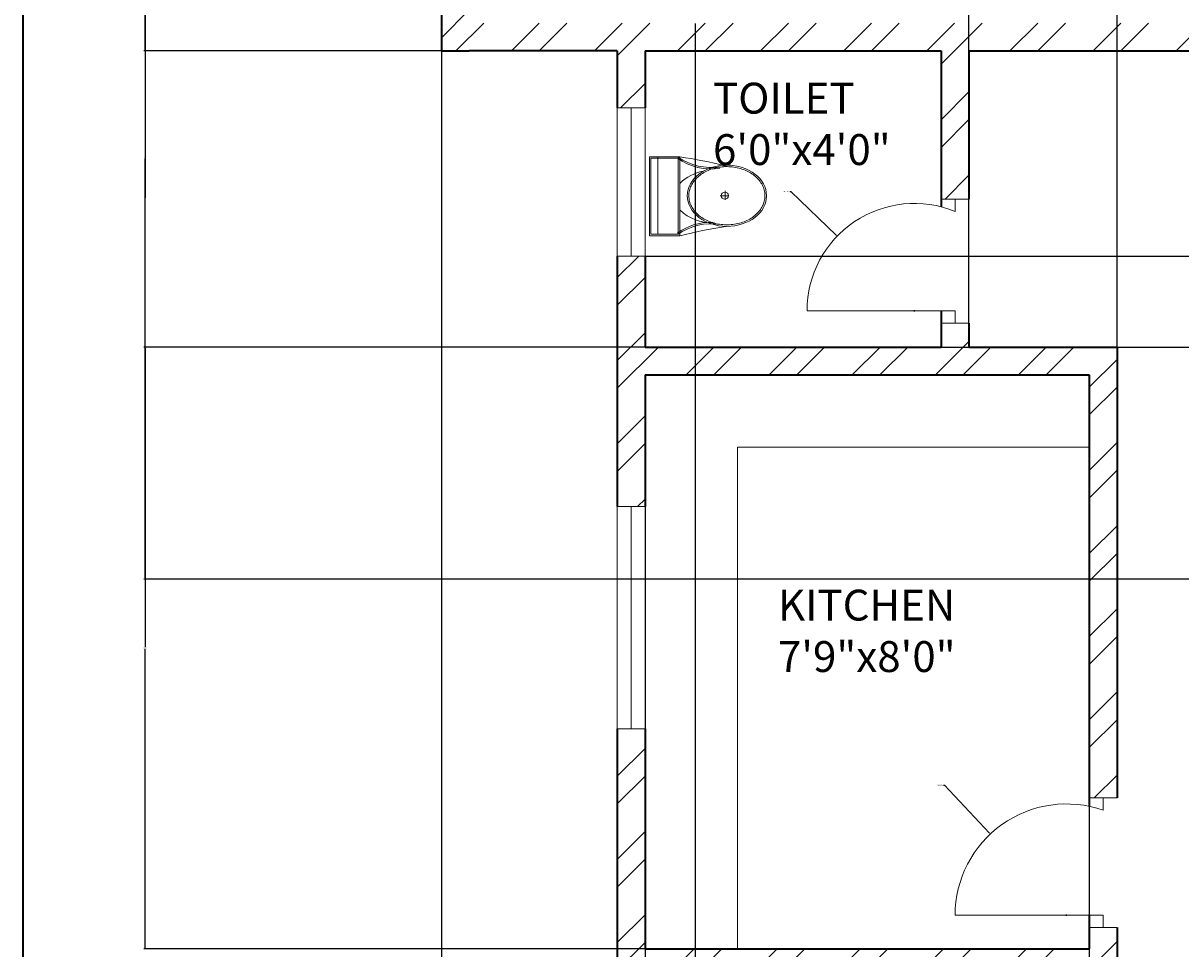
# Model space of a CAD drawing. Units: inches. Extents: x 2008 to 2657, y 1077 to 2165.
# Tile 3 of 16: x 2008 to 2196, y 1417 to 1567. Entities that reach past the tile are written whole.
import ezdxf

# ---------------------------------------------------------------- set-up
doc = ezdxf.new("R2010")
doc.units = ezdxf.units.IN
for name, color, linetype, lineweight in [('A-ANNO-DIMS', 2, 'Continuous', 18), ('A-ANNO-TTLB', 7, 'Continuous', 35), ('A-AREA-IDEN', 4, 'Continuous', 18), ('A-DOOR', 11, 'Continuous', 18), ('A-FLOR-CASE', 9, 'Continuous', 18), ('A-FLOR-FIXT', 8, 'Continuous', 18), ('A-GLAZ', 191, 'Continuous', 18), ('A-WALL', 7, 'Continuous', 35)]:
    doc.layers.add(name, color=color, linetype=linetype, lineweight=lineweight)
doc.layers.add('A-WALL-PATT', color=30, linetype='Continuous', lineweight=13, true_color=0xf8991e)
doc.styles.get("Standard").update_dxf_attribs({"font": 'arial.ttf'})
doc.dimstyles.get("Standard").update_dxf_attribs({"dimtxt": 0.18, "dimasz": 0.18, "dimexe": 0.18, "dimexo": 0.0625, "dimgap": 0.09, "dimtad": 0, "dimtih": 1, "dimtoh": 1, "dimdec": 4, "dimzin": 0, "dimdsep": 46, "dimtxsty": 'Standard', "dimcen": 0.09, "dimadec": 0, "dimazin": 0, "dimtfac": 1, "dimtdec": 4, "dimtofl": 0, "dimtmove": 0, "dimatfit": 3, "dimfxl": 1, "dimtolj": 1, "dimtzin": 0, "dimarcsym": 0})

# ---------------------------------------------------------------- blocks, each defined once
blk = doc.blocks.new('A$C31115884')
for p, q in [((283.1, 497.7), (223.4, 497.7)), ((257.5, 466.4), (257.5, 523.2)), ((0, 200), (0, 0)), ((520, 200), (0, 200)), ((10, 190), (10, 10)), ((510, 190), (10, 190)), ((510, 10), (510, 190)), ((520, 0), (520, 200)), ((510, 54.5), (0, 54.5)), ((10, 10), (510, 10)), ((0, 0), (520, 0))]:
    blk.add_line(p, q)
blk.add_circle((255.6, 496.4), 23.6)
for centre, radius, start, end in [((2777.7, -204.6), 2807, 165.4549, 171.71327), ((-294.5, 403.3), 364.7, 324.20913, 9.34987), ((-294.5, 403.3), 374.7, 324.20913, 9.34987), ((805.8, 403.3), 364.7, 170.65013, 215.79087), ((3237, 905), 2807, 188.28673, 194.5451), ((139.5, 406.2), 293.5, 315.84364, 2.65635), ((805.8, 403.3), 374.7, 179.20365, 215.79087), ((383.6, 406.2), 293.5, 190.27735, 224.15636)]:
    blk.add_arc(centre, radius, start, end)
blk.add_ellipse((256.2, 509.9), major_axis=(0, -260.7), ratio=0.772727)
blk.add_open_spline([(256.2, 259.2), (263.1, 259.2), (270, 259.7), (287.8, 262.3), (298.7, 265.1), (319.9, 273.1), (330.2, 278.4), (350.1, 291.1), (359.7, 298.7), (377.7, 315.9), (386.2, 325.5), (401.7, 346.6), (408.8, 358.1), (421.3, 382.5), (426.8, 395.5), (435.9, 422.4), (439.5, 436.4), (444.8, 465.1), (446.5, 479.7), (447.9, 509.2), (447.6, 524), (445, 553.3), (442.7, 567.8), (436.3, 596), (432.1, 609.7), (421.9, 636), (416, 648.6), (402.5, 672.1), (395, 683), (378.6, 703), (369.8, 712.1), (351.1, 728), (341.3, 734.8), (320.9, 746.2), (310.4, 750.7), (288.9, 757.3), (278, 759.4), (256, 761), (245, 760.6), (223.1, 757.2), (212.3, 754.3), (191.1, 746.1), (180.8, 740.7), (160.9, 727.8), (151.4, 720.1), (133.5, 702.7), (125.1, 693), (109.6, 671.7), (102.6, 660.2), (90.2, 635.7), (84.9, 622.7), (76, 595.6), (72.4, 581.6), (67.2, 552.9), (65.6, 538.2), (64.4, 508.8), (64.8, 494), (67.5, 464.7), (69.9, 450.2), (76.6, 422), (80.8, 408.3), (91.1, 382.2), (97.2, 369.7), (110.8, 346.3), (118.4, 335.4), (134.8, 315.6), (143.7, 306.7), (162.4, 290.9), (172.3, 284.2), (192.8, 273), (203.3, 268.6), (224.8, 262.2), (235.8, 260.2), (249.9, 259.3), (253, 259.2), (256.2, 259.2)], degree=3, knots=[0, 0, 0, 0, 0.110105, 0.110105, 0.285049, 0.285049, 0.459994, 0.459994, 0.634938, 0.634938, 0.809882, 0.809882, 0.984827, 0.984827, 1.159771, 1.159771, 1.334715, 1.334715, 1.50966, 1.50966, 1.684604, 1.684604, 1.859549, 1.859549, 2.034493, 2.034493, 2.209437, 2.209437, 2.384382, 2.384382, 2.559326, 2.559326, 2.73427, 2.73427, 2.909215, 2.909215, 3.084159, 3.084159, 3.259103, 3.259103, 3.434048, 3.434048, 3.608992, 3.608992, 3.783936, 3.783936, 3.958881, 3.958881, 4.133825, 4.133825, 4.30877, 4.30877, 4.483714, 4.483714, 4.658658, 4.658658, 4.833603, 4.833603, 5.008547, 5.008547, 5.183491, 5.183491, 5.358436, 5.358436, 5.53338, 5.53338, 5.708324, 5.708324, 5.883269, 5.883269, 6.058213, 6.058213, 6.233158, 6.233158, 6.283185, 6.283185, 6.283185, 6.283185])
blk = doc.blocks.new('WIN-24IN-B')
for p, q in [((0, 24), (4.5, 24)), ((0, 24), (0, 0)), ((4.5, 24), (2.25, 24)), ((2.25, 24), (2.25, 0)), ((4.5, 0), (4.5, 24)), ((2.25, 0), (0, 0)), ((0, 0), (4.5, 0))]:
    blk.add_line(p, q)
blk = doc.blocks.new('WIN-36IN-B')
for p, q in [((0, 36), (4.5, 36)), ((0, 0), (0, 36)), ((4.5, 36), (2.25, 36)), ((2.25, 36), (2.25, 0)), ((4.5, 36), (4.5, 0)), ((2.25, 0), (0, 0)), ((0, 0), (4.5, 0))]:
    blk.add_line(p, q)
blk = doc.blocks.new('*D31')
at = {"layer": 'A-ANNO-DIMS', "color": 0, "lineweight": -2, "transparency": 16777216}
for p, q in [((2076.26, 1562.18), (2076.26, 1140.44)), ((2576.76, 1188.61), (2576.76, 1140.44)), ((2076.44, 1140.62), (2326.12, 1140.62)), ((2576.58, 1140.62), (2326.91, 1140.62))]:
    blk.add_line(p, q, dxfattribs=at)
at = {"layer": 'A-ANNO-DIMS', "color": 0, "transparency": 16777216}
for points in [[(2076.44, 1140.65), (2076.44, 1140.59), (2076.26, 1140.62)], [(2576.58, 1140.65), (2576.58, 1140.59), (2576.76, 1140.62)]]:
    blk.add_solid(points, dxfattribs=at)
at = {"layer": 'Defpoints', "color": 0, "transparency": 16777216}
for p in [(2076.26, 1562.24), (2576.76, 1188.67), (2576.76, 1140.62)]:
    blk.add_point(p, dxfattribs=at)
at = {"layer": 'A-ANNO-DIMS', "color": 0, "transparency": 16777216, "insert": (2326.51, 1140.62), "char_height": 0.18, "attachment_point": 5}
blk.add_mtext('\\A1;500.5', dxfattribs=at)
blk = doc.blocks.new('*D41')
at = {"layer": 'A-ANNO-DIMS', "color": 0, "lineweight": -2, "transparency": 16777216}
for p, q in [((2109.2, 1514.24), (2028.03, 1514.24)), ((2028.21, 1514.06), (2028.21, 1465.67)), ((2028.21, 1416.92), (2028.21, 1465.31)), ((2109.2, 1416.74), (2028.03, 1416.74))]:
    blk.add_line(p, q, dxfattribs=at)
at = {"layer": 'A-ANNO-DIMS', "color": 0, "transparency": 16777216}
for points in [[(2028.18, 1514.06), (2028.24, 1514.06), (2028.21, 1514.24)], [(2028.18, 1416.92), (2028.24, 1416.92), (2028.21, 1416.74)]]:
    blk.add_solid(points, dxfattribs=at)
at = {"layer": 'Defpoints', "color": 0, "transparency": 16777216}
for p in [(2028.21, 1514.24), (2109.26, 1514.24), (2109.26, 1416.74)]:
    blk.add_point(p, dxfattribs=at)
at = {"layer": 'A-ANNO-DIMS', "color": 0, "transparency": 16777216, "insert": (2028.21, 1465.49), "char_height": 0.18, "attachment_point": 5}
blk.add_mtext('\\A1;97.5', dxfattribs=at)
blk = doc.blocks.new('*D42')
at = {"layer": 'A-ANNO-DIMS', "color": 0, "lineweight": -2, "transparency": 16777216}
for p, q in [((2104.7, 1562.24), (2028.03, 1562.24)), ((2028.21, 1562.06), (2028.21, 1538.42)), ((2028.21, 1514.42), (2028.21, 1538.06)), ((2109.2, 1514.24), (2028.03, 1514.24))]:
    blk.add_line(p, q, dxfattribs=at)
at = {"layer": 'A-ANNO-DIMS', "color": 0, "transparency": 16777216}
for points in [[(2028.18, 1562.06), (2028.24, 1562.06), (2028.21, 1562.24)], [(2028.18, 1514.42), (2028.24, 1514.42), (2028.21, 1514.24)]]:
    blk.add_solid(points, dxfattribs=at)
at = {"layer": 'Defpoints', "color": 0, "transparency": 16777216}
for p in [(2028.21, 1562.24), (2104.76, 1562.24), (2109.26, 1514.24)]:
    blk.add_point(p, dxfattribs=at)
at = {"layer": 'A-ANNO-DIMS', "color": 0, "transparency": 16777216, "insert": (2028.21, 1538.24), "char_height": 0.18, "attachment_point": 5}
blk.add_mtext('\\A1;48', dxfattribs=at)
blk = doc.blocks.new('*D43')
at = {"layer": 'A-ANNO-DIMS', "color": 0, "lineweight": -2, "transparency": 16777216}
for p, q in [((2076.2, 1667.24), (2028.03, 1667.24)), ((2028.21, 1667.06), (2028.21, 1614.92)), ((2028.21, 1562.42), (2028.21, 1614.56)), ((2076.2, 1562.24), (2028.03, 1562.24))]:
    blk.add_line(p, q, dxfattribs=at)
at = {"layer": 'A-ANNO-DIMS', "color": 0, "transparency": 16777216}
for points in [[(2028.18, 1667.06), (2028.24, 1667.06), (2028.21, 1667.24)], [(2028.18, 1562.42), (2028.24, 1562.42), (2028.21, 1562.24)]]:
    blk.add_solid(points, dxfattribs=at)
at = {"layer": 'Defpoints', "color": 0, "transparency": 16777216}
for p in [(2028.21, 1667.24), (2076.26, 1667.24), (2076.26, 1562.24)]:
    blk.add_point(p, dxfattribs=at)
at = {"layer": 'A-ANNO-DIMS', "color": 0, "transparency": 16777216, "insert": (2028.21, 1614.74), "char_height": 0.18, "attachment_point": 5}
blk.add_mtext('\\A1;105', dxfattribs=at)
blk = doc.blocks.new('*D53')
at = {"layer": 'A-ANNO-DIMS', "color": 0, "lineweight": -2, "transparency": 16777216}
for p, q in [((2406.7, 1613.17), (2028.03, 1613.17)), ((2028.21, 1612.99), (2028.21, 1545.11)), ((2028.21, 1476.85), (2028.21, 1544.74)), ((2406.7, 1476.67), (2028.03, 1476.67))]:
    blk.add_line(p, q, dxfattribs=at)
at = {"layer": 'A-ANNO-DIMS', "color": 0, "transparency": 16777216}
for points in [[(2028.18, 1612.99), (2028.24, 1612.99), (2028.21, 1613.17)], [(2028.18, 1476.85), (2028.24, 1476.85), (2028.21, 1476.67)]]:
    blk.add_solid(points, dxfattribs=at)
at = {"layer": 'Defpoints', "color": 0, "transparency": 16777216}
for p in [(2406.76, 1613.17), (2028.21, 1476.67), (2406.76, 1476.67)]:
    blk.add_point(p, dxfattribs=at)
at = {"layer": 'A-ANNO-DIMS', "color": 0, "transparency": 16777216, "insert": (2028.21, 1544.92), "char_height": 0.18, "attachment_point": 5}
blk.add_mtext('\\A1;136.5', dxfattribs=at)
blk = doc.blocks.new('*D54')
at = {"layer": 'A-ANNO-DIMS', "color": 0, "lineweight": -2, "transparency": 16777216}
for p, q in [((2161.76, 1514.3), (2161.76, 2142.9)), ((2161.94, 2142.72), (2173.54, 2142.72)), ((2185.58, 2142.72), (2173.98, 2142.72)), ((2185.76, 1514.3), (2185.76, 2142.9))]:
    blk.add_line(p, q, dxfattribs=at)
at = {"layer": 'A-ANNO-DIMS', "color": 0, "transparency": 16777216}
for points in [[(2161.94, 2142.75), (2161.94, 2142.69), (2161.76, 2142.72)], [(2185.58, 2142.75), (2185.58, 2142.69), (2185.76, 2142.72)]]:
    blk.add_solid(points, dxfattribs=at)
at = {"layer": 'Defpoints', "color": 0, "transparency": 16777216}
for p in [(2185.76, 2142.72), (2161.76, 1514.24), (2185.76, 1514.24)]:
    blk.add_point(p, dxfattribs=at)
at = {"layer": 'A-ANNO-DIMS', "color": 0, "transparency": 16777216, "insert": (2173.76, 2142.72), "char_height": 0.18, "attachment_point": 5}
blk.add_mtext('\\A1;24', dxfattribs=at)
blk = doc.blocks.new('*D55')
at = {"layer": 'A-ANNO-DIMS', "color": 0, "lineweight": -2, "transparency": 16777216}
for p, q in [((2109.26, 1509.68), (2109.26, 1140.44)), ((2181.26, 1509.68), (2181.26, 1140.44)), ((2109.44, 1140.62), (2145.04, 1140.62)), ((2181.08, 1140.62), (2145.48, 1140.62))]:
    blk.add_line(p, q, dxfattribs=at)
at = {"layer": 'A-ANNO-DIMS', "color": 0, "transparency": 16777216}
for points in [[(2109.44, 1140.65), (2109.44, 1140.59), (2109.26, 1140.62)], [(2181.08, 1140.65), (2181.08, 1140.59), (2181.26, 1140.62)]]:
    blk.add_solid(points, dxfattribs=at)
at = {"layer": 'Defpoints', "color": 0, "transparency": 16777216}
for p in [(2109.26, 1509.74), (2181.26, 1509.74), (2109.26, 1140.62)]:
    blk.add_point(p, dxfattribs=at)
at = {"layer": 'A-ANNO-DIMS', "color": 0, "transparency": 16777216, "insert": (2145.26, 1140.62), "char_height": 0.18, "attachment_point": 5}
blk.add_mtext('\\A1;72', dxfattribs=at)
blk = doc.blocks.new('*D62')
at = {"layer": 'A-ANNO-DIMS', "color": 0, "lineweight": -2, "transparency": 16777216}
for p, q in [((2117.38, 1566.68), (2117.38, 1140.44)), ((2237.38, 1566.68), (2237.38, 1140.44)), ((2117.56, 1140.62), (2177.1, 1140.62)), ((2237.2, 1140.62), (2177.66, 1140.62))]:
    blk.add_line(p, q, dxfattribs=at)
at = {"layer": 'A-ANNO-DIMS', "color": 0, "transparency": 16777216}
for points in [[(2117.56, 1140.65), (2117.56, 1140.59), (2117.38, 1140.62)], [(2237.2, 1140.65), (2237.2, 1140.59), (2237.38, 1140.62)]]:
    blk.add_solid(points, dxfattribs=at)
at = {"layer": 'Defpoints', "color": 0, "transparency": 16777216}
for p in [(2117.38, 1566.74), (2237.38, 1566.74), (2237.38, 1140.62)]:
    blk.add_point(p, dxfattribs=at)
at = {"layer": 'A-ANNO-DIMS', "color": 0, "transparency": 16777216, "insert": (2177.38, 1140.62), "char_height": 0.18, "attachment_point": 5}
blk.add_mtext('\\A1;120', dxfattribs=at)
blk = doc.blocks.new('*D69')
at = {"layer": 'A-ANNO-DIMS', "color": 0, "lineweight": -2, "transparency": 16777216}
for p, q in [((2109.32, 1529), (2624.99, 1529)), ((2624.81, 1528.82), (2624.81, 1521.8)), ((2624.81, 1514.42), (2624.81, 1521.44)), ((2109.32, 1514.24), (2624.99, 1514.24))]:
    blk.add_line(p, q, dxfattribs=at)
at = {"layer": 'A-ANNO-DIMS', "color": 0, "transparency": 16777216}
for points in [[(2624.78, 1528.82), (2624.84, 1528.82), (2624.81, 1529)], [(2624.78, 1514.42), (2624.84, 1514.42), (2624.81, 1514.24)]]:
    blk.add_solid(points, dxfattribs=at)
at = {"layer": 'Defpoints', "color": 0, "transparency": 16777216}
for p in [(2109.26, 1529), (2624.81, 1529), (2109.26, 1514.24)]:
    blk.add_point(p, dxfattribs=at)
at = {"layer": 'A-ANNO-DIMS', "color": 0, "transparency": 16777216, "insert": (2624.81, 1521.62), "char_height": 0.18, "attachment_point": 5}
blk.add_mtext('\\A1;14.756', dxfattribs=at)
blk = doc.blocks.new('*D91')
at = {"layer": 'A-ANNO-DIMS', "color": 0, "lineweight": -2, "transparency": 16777216}
for p, q in [((2132.7, 1539.47), (2132.88, 1539.47)), ((2132.88, 1539.47), (2140.27, 1532.35)), ((2152.83, 1520.13), (2153.01, 1520.13)), ((2152.92, 1520.04), (2152.92, 1520.22))]:
    blk.add_line(p, q, dxfattribs=at)
at = {"layer": 'A-ANNO-DIMS', "color": 0, "transparency": 16777216}
blk.add_solid([(2140.29, 1532.37), (2140.25, 1532.32), (2140.4, 1532.22)], dxfattribs=at)
at = {"layer": 'Defpoints', "color": 0, "transparency": 16777216}
for p in [(2140.4, 1532.22), (2152.92, 1520.13)]:
    blk.add_point(p, dxfattribs=at)
at = {"layer": 'A-ANNO-DIMS', "color": 0, "transparency": 16777216, "insert": (2132.15, 1539.47), "char_height": 0.18, "attachment_point": 5}
blk.add_mtext('\\A1;R17.407', dxfattribs=at)
blk = doc.blocks.new('*D92')
at = {"layer": 'A-ANNO-DIMS', "color": 0, "lineweight": -2, "transparency": 16777216}
for p, q in [((2157.64, 1443.24), (2157.82, 1443.24)), ((2157.82, 1443.24), (2165.09, 1435.48)), ((2177.46, 1422.19), (2177.64, 1422.19)), ((2177.55, 1422.1), (2177.55, 1422.28))]:
    blk.add_line(p, q, dxfattribs=at)
at = {"layer": 'A-ANNO-DIMS', "color": 0, "transparency": 16777216}
blk.add_solid([(2165.12, 1435.5), (2165.07, 1435.46), (2165.22, 1435.35)], dxfattribs=at)
at = {"layer": 'Defpoints', "color": 0, "transparency": 16777216}
for p in [(2165.22, 1435.35), (2177.55, 1422.19)]:
    blk.add_point(p, dxfattribs=at)
at = {"layer": 'A-ANNO-DIMS', "color": 0, "transparency": 16777216, "insert": (2157.09, 1443.24), "char_height": 0.18, "attachment_point": 5}
blk.add_mtext('\\A1;R18.034', dxfattribs=at)

msp = doc.modelspace()

# ---------------------------------------------------------------- hatches: boundary and pattern name
at = {"layer": 'A-WALL-PATT'}
h = msp.add_hatch(dxfattribs=at)
h.set_pattern_fill('ANSI32', color=256)
h.paths.add_polyline_path([(2109.2619, 2094.6743), (2104.7619, 2094.6743), (2104.7619, 2072.1743), (2104.7619, 2021.6151), (2109.2619, 2021.6151), (2109.2619, 2055.6743), (2126.1387, 2055.6743), (2126.1387, 2057.9243), (2126.1387, 2060.1743), (2109.2619, 2060.1743)])
h.paths.add_polyline_path([(2223.2494, 2057.9243), (2223.2494, 2060.1743), (2186.1387, 2060.1743), (2186.1387, 2055.6743), (2223.2494, 2055.6743)])
h.paths.add_polyline_path([(2250.7619, 2072.1743), (2250.7619, 2090.1743), (2250.7619, 2094.6743), (2246.2619, 2094.6743), (2246.2619, 2060.1743), (2242.7242, 2060.1743), (2242.7242, 2055.6743), (2246.2619, 2055.6743), (2246.2619, 1899.6743), (2242.7458, 1899.6743), (2242.7458, 1897.4243), (2242.7458, 1895.1743), (2246.2619, 1895.1743), (2246.2619, 1878.8745), (2248.5119, 1878.8745), (2250.7619, 1878.8745), (2250.7619, 1991.1743), (2250.7619, 2025.6743), (2257.6798, 2025.6743), (2257.6798, 2027.9243), (2257.6798, 2030.1743), (2250.7619, 2030.1743)])
h.paths.add_polyline_path([(2411.2619, 2031.6743), (2409.0119, 2031.6743), (2406.7619, 2031.6743), (2406.7619, 2030.1743), (2322.7619, 2030.1743), (2322.7619, 2053.3443), (2318.2619, 2053.3443), (2318.2619, 2030.1743), (2305.6798, 2030.1743), (2305.6798, 2025.6743), (2318.2619, 2025.6743), (2322.7619, 2025.6743), (2406.7619, 2025.6743), (2406.7619, 1995.6743), (2406.7619, 1847.2677), (2250.7619, 1847.2677), (2250.7619, 1850.9902), (2248.5119, 1850.9902), (2246.2619, 1850.9902), (2246.2619, 1847.1743), (2246.2619, 1842.7677), (2303.0015, 1842.7677), (2303.0015, 1667.2413), (2298.4208, 1667.2413), (2298.4208, 1662.7413), (2303.0015, 1662.7413), (2303.0015, 1649.8758), (2307.5015, 1649.8758), (2307.5015, 1842.7677), (2406.7619, 1842.7677), (2411.2619, 1842.7677), (2411.2619, 1878.6743), (2415.8196, 1878.6743), (2415.8196, 1880.9243), (2415.8196, 1883.1743), (2411.2619, 1883.1743)])
h.paths.add_polyline_path([(2411.2619, 2094.6743), (2406.7619, 2094.6743), (2318.2619, 2094.6743), (2318.2619, 2077.3443), (2322.7619, 2077.3443), (2322.7619, 2090.1743), (2406.7619, 2090.1743), (2406.7619, 2072.1743), (2406.7619, 2067.6743), (2406.7619, 2052.7524), (2411.2619, 2052.7524), (2411.2619, 2055.6743), (2414.9888, 2055.6743), (2414.9888, 2057.9243), (2414.9888, 2060.1743), (2411.2619, 2060.1743), (2411.2619, 2072.1743)])
h.paths.add_polyline_path([(2576.7619, 2072.1743), (2576.7619, 2094.6743), (2572.2619, 2094.6743), (2572.2619, 2060.1743), (2525.8113, 2060.1743), (2525.8113, 2055.6743), (2572.2619, 2055.6743), (2572.2619, 1994.289), (2576.7619, 1994.289)])
h.paths.add_polyline_path([(2465.8113, 2060.1743), (2436.2802, 2060.1743), (2436.2802, 2055.6743), (2465.8113, 2055.6743), (2465.8113, 2057.9243)])
h.paths.add_polyline_path([(2576.7619, 1934.289), (2574.5119, 1934.289), (2572.2619, 1934.289), (2572.2619, 1883.1743), (2447.7027, 1883.1743), (2447.7027, 1878.6743), (2459.7619, 1878.6743), (2459.7619, 1830.4982), (2464.2619, 1830.4982), (2464.2619, 1878.6743), (2572.2619, 1878.6743), (2572.2619, 1868.4883), (2576.7619, 1868.4883)])
h.paths.add_polyline_path([(2576.7619, 1832.4883), (2572.2619, 1832.4883), (2572.2619, 1806.6743), (2464.2619, 1806.6743), (2464.2619, 1809.6629), (2459.7619, 1809.6629), (2459.7619, 1802.1743), (2483.7619, 1802.1743), (2483.7619, 1778.1743), (2488.2619, 1778.1743), (2488.2619, 1802.1743), (2572.2619, 1802.1743), (2572.2619, 1793.6101), (2576.7619, 1793.6101)])
h.paths.add_polyline_path([(2576.7619, 1769.6101), (2572.2619, 1769.6101), (2572.2619, 1754.1743), (2488.2619, 1754.1743), (2488.2619, 1757.2675), (2486.0119, 1757.2675), (2483.7619, 1757.2675), (2483.7619, 1754.1743), (2447.4528, 1754.1743), (2447.4528, 1749.6743), (2483.7619, 1749.6743), (2572.2619, 1749.6743), (2572.2619, 1715.1837), (2576.7619, 1715.1837)])
h.paths.add_polyline_path([(2576.7619, 1655.1837), (2572.2619, 1655.1837), (2572.2619, 1617.6743), (2411.2619, 1617.6743), (2411.2619, 1749.6743), (2414.2827, 1749.6743), (2414.2827, 1754.1743), (2406.7619, 1754.1743), (2406.7619, 1749.6743), (2406.7619, 1617.6743), (2307.5015, 1617.6743), (2307.5015, 1621.0007), (2305.2515, 1621.0007), (2303.0015, 1621.0007), (2303.0015, 1609.6944), (2307.5015, 1609.6944), (2307.5015, 1613.1743), (2406.7619, 1613.1743), (2406.7619, 1476.6743), (2415.532, 1476.6743), (2415.532, 1478.9243), (2415.532, 1481.1743), (2411.2619, 1481.1743), (2411.2619, 1613.1743), (2572.2619, 1613.1743), (2572.2619, 1584.6086), (2576.7619, 1584.6086)])
h.paths.add_polyline_path([(2576.7619, 1524.6086), (2572.2619, 1524.6086), (2572.2619, 1481.1743), (2483.7619, 1481.1743), (2447.5119, 1481.1743), (2447.5119, 1476.6743), (2483.7619, 1476.6743), (2483.7619, 1473.5051), (2488.2619, 1473.5051), (2488.2619, 1476.6743), (2572.2619, 1476.6743), (2572.2619, 1469.5488), (2576.7619, 1469.5488)])
h.paths.add_polyline_path([(2576.7619, 1445.5488), (2572.2619, 1445.5488), (2572.2619, 1428.6743), (2488.2619, 1428.6743), (2488.2619, 1455.6743), (2486.0119, 1455.6743), (2483.7619, 1455.6743), (2483.7619, 1428.6743), (2459.7619, 1428.6743), (2459.7619, 1422.1519), (2464.2619, 1422.1519), (2464.2619, 1424.1743), (2572.2619, 1424.1743), (2572.2619, 1407.5685), (2576.7619, 1407.5685)])
h.paths.add_polyline_path([(2576.7619, 1371.5685), (2572.2619, 1371.5685), (2572.2619, 1352.1743), (2464.2619, 1352.1743), (2464.2619, 1403.1384), (2462.0119, 1403.1384), (2459.7619, 1403.1384), (2459.7619, 1352.1743), (2446.3194, 1352.1743), (2446.3194, 1347.6743), (2572.2619, 1347.6743), (2572.2619, 1321.0291), (2576.7619, 1321.0291)])
h.paths.add_polyline_path([(2462.703, 1227.6743), (2436.0298, 1227.6743), (2436.0298, 1225.4243), (2436.0298, 1223.1743), (2462.703, 1223.1743), (2462.703, 1225.4243)])
h.paths.add_polyline_path([(2576.7619, 1261.0291), (2574.5119, 1261.0291), (2572.2619, 1261.0291), (2572.2619, 1227.6743), (2522.703, 1227.6743), (2522.703, 1223.1743), (2572.2619, 1223.1743), (2572.2619, 1188.6743), (2576.7619, 1188.6743), (2576.7619, 1193.1743), (2576.7619, 1223.1743)])
h.paths.add_polyline_path([(2414.2823, 1227.6743), (2411.2619, 1227.6743), (2411.2619, 1267.1779), (2409.0119, 1267.1779), (2406.7619, 1267.1779), (2406.7619, 1227.6743), (2322.7619, 1227.6743), (2322.7619, 1244.3623), (2318.2619, 1244.3623), (2318.2619, 1223.1743), (2406.7619, 1223.1743), (2406.7619, 1193.1743), (2406.7619, 1188.6743), (2411.2619, 1188.6743), (2411.2619, 1193.1743), (2411.2619, 1223.1743), (2414.2823, 1223.1743)])
h.paths.add_polyline_path([(2411.2619, 1347.6743), (2414.702, 1347.6743), (2414.702, 1349.9243), (2414.702, 1352.1743), (2411.2619, 1352.1743), (2411.2619, 1416.7413), (2307.5015, 1416.7413), (2307.5015, 1579.8489), (2305.2515, 1579.8489), (2303.0015, 1579.8489), (2303.0015, 1566.7413), (2299.2719, 1566.7413), (2299.2719, 1562.2413), (2303.0015, 1562.2413), (2303.0015, 1416.7413), (2246.2619, 1416.7413), (2246.2619, 1409.8616), (2250.7619, 1409.8616), (2250.7619, 1412.2413), (2406.7619, 1412.2413), (2406.7619, 1292.1743), (2304.9703, 1292.1743), (2304.9703, 1287.6743), (2318.2619, 1287.6743), (2318.2619, 1268.3623), (2322.7619, 1268.3623), (2322.7619, 1287.6743), (2406.7619, 1287.6743), (2406.7619, 1285.4748), (2411.2619, 1285.4748)])
h.paths.add_polyline_path([(2109.2619, 1262.7482), (2104.7619, 1262.7482), (2104.7619, 1223.1743), (2104.7619, 1193.1743), (2104.7619, 1188.6743), (2109.2619, 1188.6743), (2109.2619, 1223.1743), (2126.7928, 1223.1743), (2126.7928, 1225.4243), (2126.7928, 1227.6743), (2109.2619, 1227.6743)])
h.paths.add_polyline_path([(2222.3268, 1227.6743), (2186.7928, 1227.6743), (2186.7928, 1223.1743), (2222.3268, 1223.1743)])
h.paths.add_polyline_path([(2250.7619, 1287.6743), (2256.9703, 1287.6743), (2256.9703, 1289.9243), (2256.9703, 1292.1743), (2250.7619, 1292.1743), (2250.7619, 1382.2078), (2248.5119, 1382.2078), (2246.2619, 1382.2078), (2246.2619, 1347.6743), (2246.2619, 1227.6743), (2242.6068, 1227.6743), (2242.6068, 1223.1743), (2246.2619, 1223.1743), (2246.2619, 1188.6743), (2250.7619, 1188.6743), (2250.7619, 1193.1743), (2250.7619, 1227.6743)])
h.paths.add_polyline_path([(2133.2619, 1349.9243), (2133.2619, 1352.1743), (2109.2619, 1352.1743), (2109.2619, 1375.2826), (2104.7619, 1375.2826), (2104.7619, 1322.7482), (2109.2619, 1322.7482), (2109.2619, 1347.6743), (2133.2619, 1347.6743)])
h.paths.add_polyline_path([(2210.2105, 1352.1743), (2161.7619, 1352.1743), (2161.7619, 1412.2413), (2185.7619, 1412.2413), (2185.7619, 1420.1851), (2183.5119, 1420.1851), (2181.2619, 1420.1851), (2181.2619, 1416.7413), (2109.2619, 1416.7413), (2109.2619, 1452.4006), (2104.7619, 1452.4006), (2104.7619, 1399.2826), (2109.2619, 1399.2826), (2109.2619, 1412.2413), (2157.2619, 1412.2413), (2157.2619, 1352.1743), (2154.3383, 1352.1743), (2154.3383, 1347.6743), (2210.2105, 1347.6743)])
h.paths.add_polyline_path([(2185.7619, 1514.2413), (2161.7619, 1514.2413), (2161.7619, 1518.1307), (2159.5119, 1518.1307), (2157.2619, 1518.1307), (2157.2619, 1514.2413), (2109.2619, 1514.2413), (2109.2619, 1528.997), (2107.0119, 1528.997), (2104.7619, 1528.997), (2104.7619, 1488.4006), (2109.2619, 1488.4006), (2109.2619, 1509.7413), (2181.2619, 1509.7413), (2181.2619, 1441.2042), (2185.7619, 1441.2042)])
h.paths.add_polyline_path([(2270.4025, 1566.7413), (2109.2619, 1566.7413), (2080.7619, 1566.7413), (2080.7619, 1586.5643), (2076.2619, 1586.5643), (2076.2619, 1562.2413), (2080.7619, 1562.2413), (2104.7619, 1562.2413), (2104.7619, 1552.997), (2109.2619, 1552.997), (2109.2619, 1562.2413), (2157.2619, 1562.2413), (2157.2619, 1538.2413), (2161.7619, 1538.2413), (2161.7619, 1562.2413), (2205.2619, 1562.2413), (2270.4025, 1562.2413)])
h.paths.add_polyline_path([(2131.6813, 1897.4243), (2131.6813, 1899.6743), (2109.2619, 1899.6743), (2109.2619, 1961.6151), (2104.7619, 1961.6151), (2104.7619, 1886.8042), (2109.2619, 1886.8042), (2109.2619, 1895.1743), (2131.6813, 1895.1743)])
h.paths.add_polyline_path([(2185.7619, 1847.1743), (2161.7619, 1847.1743), (2161.7619, 1895.1743), (2185.7619, 1895.1743), (2211.543, 1895.1743), (2211.543, 1897.4243), (2211.543, 1899.6743), (2154.0916, 1899.6743), (2154.0916, 1897.4243), (2154.0916, 1895.1743), (2157.2619, 1895.1743), (2157.2619, 1847.1743), (2109.2619, 1847.1743), (2109.2619, 1862.8042), (2104.7619, 1862.8042), (2104.7619, 1821.243), (2109.2619, 1821.243), (2109.2619, 1842.6743), (2181.2619, 1842.6743), (2181.2619, 1840.6763), (2185.7619, 1840.6763)])
h.paths.add_polyline_path([(2109.2619, 1785.243), (2104.7619, 1785.243), (2104.7619, 1715.4691), (2109.2619, 1715.4691), (2109.2619, 1730.8423), (2157.2619, 1730.8423), (2157.2619, 1727.6404), (2161.7619, 1727.6404), (2161.7619, 1730.8423), (2185.7619, 1730.8423), (2185.7619, 1822.1438), (2183.5119, 1822.1438), (2181.2619, 1822.1438), (2181.2619, 1735.3423), (2109.2619, 1735.3423)])
h.paths.add_polyline_path([(2109.2619, 1691.4691), (2104.7619, 1691.4691), (2104.7619, 1667.2413), (2076.2619, 1667.2413), (2076.2619, 1646.5643), (2080.7619, 1646.5643), (2080.7619, 1662.7413), (2109.2619, 1662.7413), (2271.4941, 1662.7413), (2271.4941, 1664.9913), (2271.4941, 1667.2413), (2181.2619, 1667.2413), (2161.7619, 1667.2413), (2161.7619, 1708.3752), (2159.5119, 1708.3752), (2157.2619, 1708.3752), (2157.2619, 1667.2413), (2109.2619, 1667.2413)])
h.paths.add_polyline_path([(2233.1467, 1747.4973), (2270.0737, 1747.4973), (2270.0737, 1766.1547), (2233.1467, 1766.1547)], flags=9)

# ---------------------------------------------------------------- linework, layer by layer
at = {"layer": 'A-ANNO-TTLB'}
msp.add_lwpolyline([(2008.4537, 2164.5615), (2657.4477, 2164.5615), (2657.4477, 1076.8888), (2008.4537, 1076.8888)], close=True, dxfattribs=at)
at = {"layer": 'A-DOOR'}
for p, q in [((2157.2619, 1538.2413), (2161.7619, 1538.2413)), ((2161.7619, 1538.2413), (2159.5119, 1538.2413)), ((2159.5119, 1538.2413), (2159.5119, 1536.2413)), ((2159.5119, 1520.1307), (2135.5119, 1520.1307)), ((2159.5119, 1518.1307), (2159.5119, 1520.1307)), ((2157.2619, 1518.1307), (2161.7619, 1518.1307)), ((2161.7619, 1518.1307), (2159.5119, 1518.1307)), ((2181.2619, 1441.2042), (2185.7619, 1441.2042)), ((2185.7619, 1441.2042), (2183.5119, 1441.2042)), ((2183.5119, 1441.2042), (2183.5119, 1439.2042)), ((2183.5119, 1422.1851), (2159.5119, 1422.1851)), ((2183.5119, 1420.1851), (2183.5119, 1422.1851)), ((2181.2619, 1420.1851), (2185.7619, 1420.1851)), ((2185.7619, 1420.1851), (2183.5119, 1420.1851))]:
    msp.add_line(p, q, dxfattribs=at)
for centre, radius, start in [((2152.9192, 1520.1307), 17.4073, 67.744942), ((2177.5463, 1422.1851), 18.0344, 70.683168)]:
    msp.add_arc(centre, radius, start, 180, dxfattribs=at)
at = {"layer": 'A-FLOR-CASE'}
for p, q in [((2124.2222, 1416.7413), (2124.2222, 1498.0524)), ((2124.2222, 1498.0524), (2181.2619, 1498.0524))]:
    msp.add_line(p, q, dxfattribs=at)
at = {"layer": 'A-WALL'}
for p, q in [((2076.2619, 1586.5643), (2076.2619, 1562.2413)), ((2076.2619, 1562.2413), (2080.7619, 1562.2413)), ((2104.7619, 1562.2413), (2080.7619, 1562.2413)), ((2104.7619, 1562.2413), (2104.7619, 1552.997)), ((2109.2619, 1562.2413), (2157.2619, 1562.2413)), ((2109.2619, 1562.2413), (2109.2619, 1552.997)), ((2109.2619, 1562.2413), (2157.2619, 1562.2413)), ((2157.2619, 1562.2413), (2157.2619, 1536.9877)), ((2161.7619, 1562.2413), (2161.7619, 1538.2413)), ((2161.7619, 1562.2413), (2271.6639, 1562.2413)), ((2161.7619, 1562.2413), (2205.2619, 1562.2413)), ((2104.7619, 1528.997), (2104.7619, 1488.4006)), ((2109.2619, 1528.997), (2109.2619, 1514.2413)), ((2157.2619, 1520.1307), (2157.2619, 1514.2413)), ((2161.7619, 1518.1307), (2161.7619, 1514.2413)), ((2109.2619, 1514.2413), (2157.2619, 1514.2413)), ((2161.7619, 1514.2413), (2185.7619, 1514.2413)), ((2185.7619, 1514.2413), (2185.7619, 1441.2042)), ((2109.2619, 1509.7413), (2181.2619, 1509.7413)), ((2109.2619, 1509.7413), (2109.2619, 1488.4006)), ((2181.2619, 1509.7413), (2181.2619, 1439.8326)), ((2104.7619, 1452.4006), (2104.7619, 1399.2826)), ((2109.2619, 1452.4006), (2109.2619, 1416.7413)), ((2181.2619, 1422.1851), (2181.2619, 1416.7413)), ((2185.7619, 1420.1851), (2185.7619, 1412.2413)), ((2109.2619, 1416.7413), (2181.2619, 1416.7413))]:
    msp.add_line(p, q, dxfattribs=at)

# ---------------------------------------------------------------- block references
at = {"layer": 'A-FLOR-FIXT', "xscale": 0.0246256636748975, "yscale": 0.0246256636748975, "zscale": 0.0246256636748975, "rotation": 270}
msp.add_blockref('A$C31115884', (2109.9696, 1545.0846), dxfattribs=at)
at = {"layer": 'A-GLAZ', "rotation": 180}
msp.add_blockref('WIN-24IN-B', (2109.2618, 1552.9973), dxfattribs=at)
at = {"layer": 'A-GLAZ'}
msp.add_blockref('WIN-36IN-B', (2104.762, 1452.401), dxfattribs=at)

# ---------------------------------------------------------------- texts
at = {"layer": 'A-AREA-IDEN', "char_height": 5, "attachment_point": 1}
for s, width, insert in [('TOILET\\P6\'0"x4\'0"', 47.213094, (2120.2737, 1557.0909)), ('KITCHEN\\P7\'9"x8\'0"', 162.381017, (2130.8005, 1474.9381))]:
    msp.add_mtext_dynamic_manual_height_columns(s, width=width, gutter_width=12.5, heights=[0], dxfattribs=dict(at, insert=insert))

# ---------------------------------------------------------------- dimensions: what is measured, and where the dimension line sits
at = {"layer": 'A-ANNO-DIMS'}
for base, p1, p2, override, picture, middle in [((2185.7619, 2142.7243), (2161.7619, 1514.2413), (2185.7619, 1514.2413), {"dimdec": 0, "dimlfac": 1, "dimrnd": 0, "dimzin": 0, "dimdsep": 46, "dimlunit": 2}, '*D54', (2173.7619, 2142.7243)), ((2237.3789, 1140.6243), (2117.3789, 1566.7413), (2237.3789, 1566.7413), {"dimdec": 0, "dimlfac": 1, "dimrnd": 0, "dimzin": 0, "dimdsep": 46, "dimlunit": 2}, '*D62', (2177.3789, 1140.6243)), ((2576.7619, 1140.6243), (2076.2619, 1562.2413), (2576.7619, 1188.6743), {"dimdec": 1, "dimlfac": 1, "dimrnd": 0, "dimzin": 0, "dimdsep": 46, "dimlunit": 2}, '*D31', (2326.5119, 1140.6243)), ((2109.2619, 1140.6243), (2181.2619, 1509.7413), (2109.2619, 1509.7413), {"dimdec": 0, "dimlfac": 1, "dimrnd": 0, "dimzin": 0, "dimdsep": 46, "dimlunit": 2}, '*D55', (2145.2619, 1140.6243))]:
    dim = msp.add_linear_dim(base=base, p1=p1, p2=p2, dimstyle='Standard', override=override, dxfattribs=at)
    dim.commit()
    dim.dimension.update_dxf_attribs({"geometry": picture, "text_midpoint": middle})
for base, p1, p2, override, picture, middle in [((2028.2119, 1667.2413), (2076.2619, 1562.2413), (2076.2619, 1667.2413), {"dimdec": 0, "dimlfac": 1, "dimrnd": 0, "dimzin": 0, "dimdsep": 46, "dimlunit": 2}, '*D43', (2028.2119, 1614.7413)), ((2028.2119, 1476.6743), (2406.7619, 1613.1743), (2406.7619, 1476.6743), {"dimdec": 1, "dimlfac": 1, "dimrnd": 0, "dimzin": 0, "dimdsep": 46, "dimlunit": 2}, '*D53', (2028.2119, 1544.9243)), ((2028.2119, 1562.2413), (2109.2619, 1514.2413), (2104.7619, 1562.2413), {"dimdec": 0, "dimlfac": 1, "dimrnd": 0, "dimzin": 0, "dimdsep": 46, "dimlunit": 2}, '*D42', (2028.2119, 1538.2413)), ((2624.8119, 1528.997), (2109.2619, 1514.2413), (2109.2619, 1528.997), {"dimdec": 3, "dimlfac": 1, "dimrnd": 0, "dimzin": 0, "dimdsep": 46, "dimlunit": 2}, '*D69', (2624.8119, 1521.6192)), ((2028.2119, 1514.2413), (2109.2619, 1416.7413), (2109.2619, 1514.2413), {"dimdec": 1, "dimlfac": 1, "dimrnd": 0, "dimzin": 0, "dimdsep": 46, "dimlunit": 2}, '*D41', (2028.2119, 1465.4913))]:
    dim = msp.add_linear_dim(base=base, p1=p1, p2=p2, angle=90, dimstyle='Standard', override=override, dxfattribs=at)
    dim.commit()
    dim.dimension.update_dxf_attribs({"geometry": picture, "text_midpoint": middle})
for center, mpoint, picture, middle in [((2152.9192, 1520.1307), (2140.3955, 1532.2209), '*D91', (2132.1515, 1539.475)), ((2177.5463, 1422.1851), (2165.2162, 1435.346), '*D92', (2157.0888, 1443.2425))]:
    dim = msp.add_radius_dim(center=center, mpoint=mpoint, dimstyle='Standard', override={"dimdec": 3, "dimlfac": 1, "dimrnd": 0, "dimzin": 0, "dimdsep": 46, "dimlunit": 2}, dxfattribs=at)
    dim.commit()
    dim.dimension.update_dxf_attribs({"geometry": picture, "text_midpoint": middle, "dimtype": 164})

doc.saveas('drawing.dxf')
